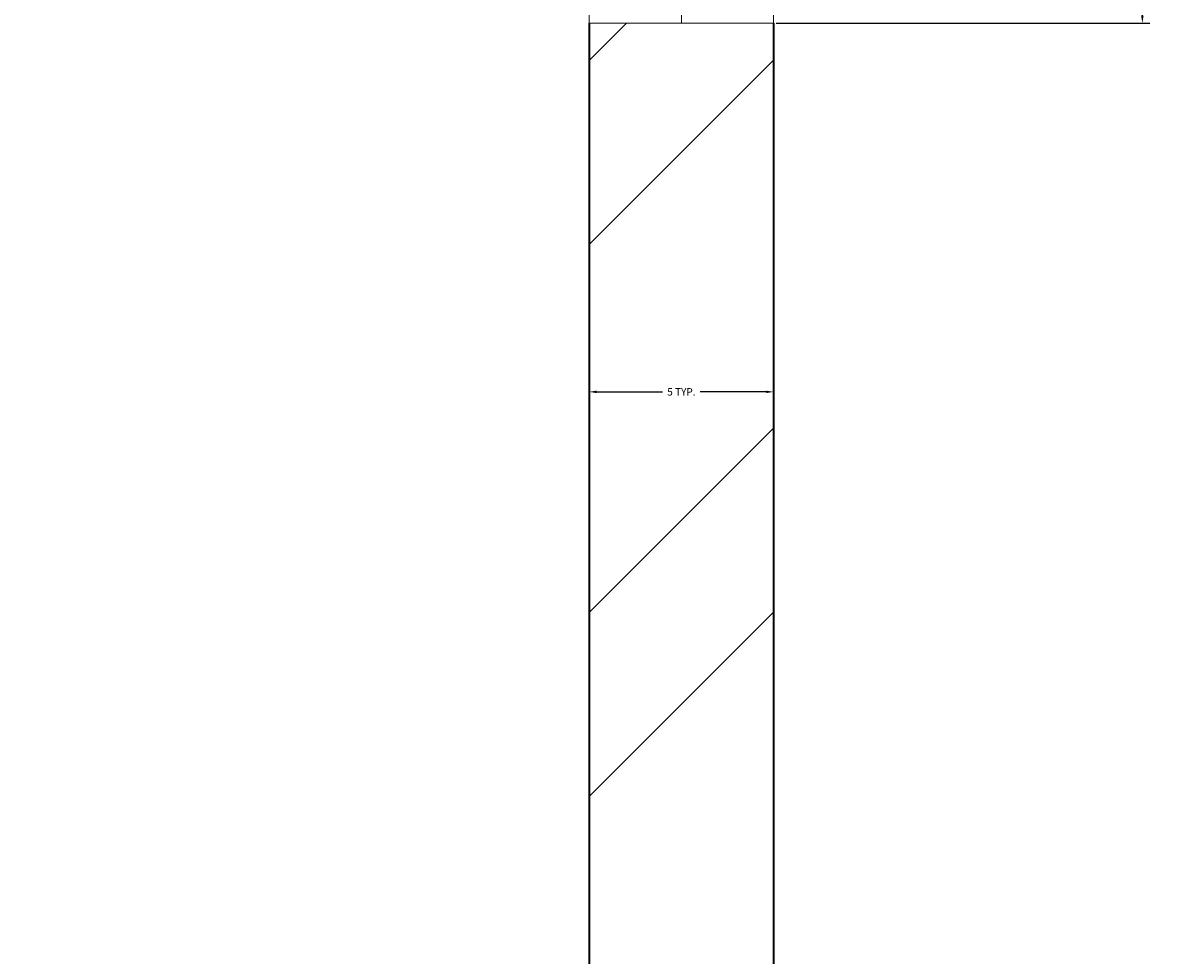
# Model space of a CAD drawing. Units: inches. Extents: x 2168 to 3056, y 1130 to 2629.
# Tile 41 of 42: x 2846 to 2874, y 2286 to 2308. Entities that reach past the tile are written whole.
import ezdxf

# ---------------------------------------------------------------- set-up
doc = ezdxf.new("R2010")
doc.units = ezdxf.units.IN
for name, color, linetype, lineweight in [('A-ANNO-DIMS', 2, 'Continuous', 18), ('A-GLAZ', 201, 'Continuous', 18), ('A-WALL', 7, 'Continuous', 35)]:
    doc.layers.add(name, color=color, linetype=linetype, lineweight=lineweight)
doc.layers.add('A-WALL-PATT', color=143, linetype='Continuous', lineweight=13, true_color=0x7aafdf)
doc.styles.get("Standard").update_dxf_attribs({"font": 'arial.ttf'})
doc.dimstyles.get("Standard").update_dxf_attribs({"dimtxt": 0.18, "dimasz": 0.18, "dimexe": 0.18, "dimexo": 0.0625, "dimgap": 0.09, "dimtad": 0, "dimtih": 1, "dimtoh": 1, "dimdec": 4, "dimzin": 0, "dimdsep": 46, "dimtxsty": 'Standard', "dimcen": 0.09, "dimadec": 0, "dimazin": 0, "dimtfac": 1, "dimtdec": 4, "dimtofl": 0, "dimtmove": 0, "dimatfit": 3, "dimfxl": 1, "dimtolj": 1, "dimtzin": 0, "dimarcsym": 0})

# ---------------------------------------------------------------- blocks, each defined once
blk = doc.blocks.new('WIN-60')
for p, q in [((0, 0), (0, 60)), ((2.25, 0), (2.25, 60)), ((4.5, 60), (4.5, 0)), ((0, 0), (4.5, 0)), ((4.5, 0), (2.25, 0))]:
    blk.add_line(p, q)
blk = doc.blocks.new('*D38')
at = {"layer": 'A-ANNO-DIMS', "color": 0, "lineweight": -2, "transparency": 16777216}
for p, q in [((2864.358, 2368.425), (2873.476, 2368.425)), ((2873.296, 2368.245), (2873.296, 2338.609)), ((2873.296, 2308.605), (2873.296, 2338.242)), ((2864.358, 2308.425), (2873.476, 2308.425))]:
    blk.add_line(p, q, dxfattribs=at)
at = {"layer": 'A-ANNO-DIMS', "color": 0, "transparency": 16777216}
for points in [[(2873.266, 2368.245), (2873.326, 2368.245), (2873.296, 2368.425)], [(2873.266, 2308.605), (2873.326, 2308.605), (2873.296, 2308.425)]]:
    blk.add_solid(points, dxfattribs=at)
at = {"layer": 'Defpoints', "color": 0, "transparency": 16777216}
for p in [(2864.296, 2368.425), (2873.296, 2368.425), (2864.296, 2308.425)]:
    blk.add_point(p, dxfattribs=at)
at = {"layer": 'A-ANNO-DIMS', "color": 0, "transparency": 16777216, "insert": (2873.296, 2338.425), "char_height": 0.18, "attachment_point": 5}
blk.add_mtext('\\A1;WINDOW 60 TYP.', dxfattribs=at)
blk = doc.blocks.new('*D39')
at = {"layer": 'A-ANNO-DIMS', "color": 0, "lineweight": -2, "transparency": 16777216}
for p, q in [((2859.796, 2308.363), (2859.796, 2299.245)), ((2864.296, 2308.363), (2864.296, 2299.245)), ((2859.976, 2299.425), (2861.588, 2299.425)), ((2864.116, 2299.425), (2862.504, 2299.425))]:
    blk.add_line(p, q, dxfattribs=at)
at = {"layer": 'A-ANNO-DIMS', "color": 0, "transparency": 16777216}
for points in [[(2859.976, 2299.455), (2859.976, 2299.395), (2859.796, 2299.425)], [(2864.116, 2299.455), (2864.116, 2299.395), (2864.296, 2299.425)]]:
    blk.add_solid(points, dxfattribs=at)
at = {"layer": 'Defpoints', "color": 0, "transparency": 16777216}
for p in [(2859.796, 2308.425), (2864.296, 2308.425), (2864.296, 2299.425)]:
    blk.add_point(p, dxfattribs=at)
at = {"layer": 'A-ANNO-DIMS', "color": 0, "transparency": 16777216, "insert": (2862.046, 2299.425), "char_height": 0.18, "attachment_point": 5}
blk.add_mtext('\\A1;5 TYP.', dxfattribs=at)

msp = doc.modelspace()

# ---------------------------------------------------------------- hatches: boundary and pattern name
at = {"layer": 'A-WALL-PATT'}
h = msp.add_hatch(dxfattribs=at)
h.set_pattern_fill('ANSI32', color=256)
h.paths.add_polyline_path([(2463.796, 2409.389), (2467.387, 2409.389), (2467.387, 2413.889), (2454.768, 2413.889), (2454.768, 2411.639), (2454.768, 2409.389), (2459.296, 2409.389), (2459.296, 2265.389), (2455.644, 2265.389), (2455.644, 2260.889), (2467.349, 2260.889), (2467.349, 2263.139), (2467.349, 2265.389), (2463.796, 2265.389)])
h.paths.add_polyline_path([(2431.596, 2413.889), (2409.647, 2413.889), (2409.647, 2409.389), (2431.596, 2409.389), (2431.596, 2411.639)])
h.paths.add_polyline_path([(2349.647, 2413.889), (2331.796, 2413.889), (2331.796, 2362.671), (2336.296, 2362.671), (2336.296, 2409.389), (2349.647, 2409.389), (2349.647, 2411.639)])
h.paths.add_polyline_path([(2634.149, 2411.639), (2634.149, 2413.889), (2562.293, 2413.889), (2562.293, 2409.389), (2595.796, 2409.389), (2595.796, 2280.309), (2595.826, 2280.309), (2595.826, 2265.389), (2499.91, 2265.389), (2499.91, 2260.889), (2550.796, 2260.889), (2550.796, 2117.308), (2555.296, 2117.308), (2555.296, 2168.08), (2571.93, 2168.08), (2571.93, 2176.889), (2559.796, 2176.889), (2559.796, 2256.389), (2640.796, 2256.389), (2640.796, 2176.889), (2626.428, 2176.889), (2626.428, 2168.08), (2645.296, 2168.08), (2645.296, 2116.637), (2649.796, 2116.637), (2649.796, 2260.889), (2691.251, 2260.889), (2691.251, 2263.139), (2691.251, 2265.389), (2670.655, 2265.389), (2670.655, 2265.365), (2600.296, 2265.365), (2600.296, 2280.258), (2600.296, 2409.389), (2634.149, 2409.389)])
h.paths.add_polyline_path([(2600.296, 2473.889), (2612.84, 2473.889), (2612.84, 2478.389), (2572.636, 2478.389), (2572.636, 2473.889), (2595.796, 2473.889), (2595.796, 2413.889), (2600.296, 2413.889)])
h.paths.add_polyline_path([(2535.796, 2473.889), (2548.636, 2473.889), (2548.636, 2478.389), (2531.396, 2478.389), (2531.396, 2413.889), (2521.6, 2413.889), (2521.6, 2409.389), (2539.239, 2409.389), (2539.239, 2411.639), (2539.239, 2413.889), (2535.796, 2413.889)])
h.paths.add_polyline_path([(2664.796, 2478.389), (2636.84, 2478.389), (2636.84, 2473.889), (2660.296, 2473.889), (2660.296, 2413.889), (2656.165, 2413.889), (2656.165, 2409.389), (2671.684, 2409.389), (2671.684, 2411.639), (2671.684, 2413.889), (2664.796, 2413.889)])
h.paths.add_polyline_path([(2705.942, 2413.889), (2695.684, 2413.889), (2695.684, 2409.389), (2705.942, 2409.389)])
h.paths.add_polyline_path([(2741.35, 2413.889), (2728.733, 2413.889), (2728.733, 2411.639), (2728.733, 2409.389), (2732.296, 2409.389), (2732.296, 2265.389), (2725.733, 2265.389), (2725.733, 2260.889), (2740.917, 2260.889), (2740.917, 2263.139), (2740.917, 2265.389), (2736.796, 2265.389), (2736.796, 2409.389), (2741.35, 2409.389)])
h.paths.add_polyline_path([(2785.655, 2413.889), (2764.546, 2413.889), (2764.486, 2409.389), (2785.655, 2409.389), (2785.655, 2411.639)])
h.paths.add_polyline_path([(2864.296, 2413.889), (2845.655, 2413.889), (2845.655, 2409.389), (2859.796, 2409.389), (2859.796, 2368.425), (2864.296, 2368.425)])
h.paths.add_polyline_path([(2864.296, 2308.425), (2862.046, 2308.425), (2859.796, 2308.425), (2859.796, 2265.389), (2774.483, 2265.389), (2774.483, 2263.139), (2774.483, 2260.889), (2781.796, 2260.889), (2781.796, 2226.654), (2786.296, 2226.654), (2786.296, 2260.889), (2859.796, 2260.889), (2859.796, 2241.352), (2864.296, 2241.352)])
h.paths.add_polyline_path([(2864.296, 2217.352), (2862.046, 2217.352), (2859.796, 2217.352), (2859.796, 2200.889), (2786.296, 2200.889), (2786.296, 2205.931), (2784.046, 2205.931), (2781.796, 2205.931), (2781.796, 2150.974), (2786.296, 2150.974), (2786.296, 2161.889), (2859.796, 2161.889), (2859.796, 2144.419), (2864.296, 2144.419)])
h.paths.add_polyline_path([(2859.796, 2196.389), (2859.796, 2166.389), (2786.296, 2166.389), (2786.296, 2196.389)], flags=16)
h.paths.add_polyline_path([(2864.296, 2108.419), (2862.046, 2108.419), (2859.796, 2108.419), (2859.796, 2080.889), (2786.296, 2080.889), (2786.296, 2111.993), (2781.796, 2111.993), (2781.796, 2080.889), (2649.796, 2080.889), (2649.796, 2086.036), (2647.546, 2086.036), (2645.296, 2086.036), (2645.296, 2071.739), (2649.796, 2071.739), (2649.796, 2076.389), (2781.796, 2076.389), (2781.796, 2041.792), (2786.296, 2041.792), (2786.296, 2076.389), (2859.796, 2076.389), (2859.796, 2058.577), (2864.296, 2058.577)])
h.paths.add_polyline_path([(2864.296, 2022.577), (2859.796, 2022.577), (2859.796, 1992.389), (2786.296, 1992.389), (2786.296, 1999.573), (2781.796, 1999.573), (2781.796, 1848.085), (2784.046, 1848.085), (2786.296, 1848.085), (2786.296, 1851.389), (2859.796, 1851.389), (2859.796, 1838.258), (2864.296, 1838.258)], flags=17)
h.paths.add_polyline_path([(2859.796, 1987.889), (2859.796, 1855.889), (2786.296, 1855.889), (2786.296, 1987.889)], flags=16)
h.paths.add_polyline_path([(2823.046, 1987.889), (2841.421, 1921.889), (2823.046, 1855.889)], flags=0)
h.paths.add_polyline_path([(2864.296, 1814.258), (2859.796, 1814.258), (2859.796, 1791.389), (2786.296, 1791.389), (2786.296, 1825.658), (2784.046, 1825.658), (2781.796, 1825.658), (2781.796, 1791.389), (2720.155, 1791.389), (2720.155, 1791.265), (2649.796, 1791.265), (2649.796, 1806.159), (2649.796, 2038.983), (2647.546, 2038.983), (2645.296, 2038.983), (2645.296, 1783.925), (2649.796, 1783.925), (2649.796, 1786.889), (2781.796, 1786.889), (2781.796, 1746.789), (2786.296, 1746.789), (2786.296, 1786.889), (2859.796, 1786.889), (2859.796, 1770.083), (2864.296, 1770.083)])
h.paths.add_polyline_path([(2864.296, 1734.083), (2862.046, 1734.083), (2859.796, 1734.083), (2859.796, 1705.889), (2786.296, 1705.889), (2786.296, 1714.166), (2781.796, 1714.166), (2781.796, 1660.527), (2786.296, 1660.527), (2786.296, 1666.889), (2859.796, 1666.889), (2859.796, 1648.342), (2864.296, 1648.342)])
h.paths.add_polyline_path([(2786.296, 1701.389), (2859.796, 1701.389), (2859.796, 1671.389), (2786.296, 1671.389)], flags=16)
h.paths.add_polyline_path([(2649.796, 1756.576), (2647.546, 1756.576), (2645.296, 1756.576), (2645.296, 1606.889), (2555.296, 1606.889), (2555.296, 1749.513), (2553.046, 1749.513), (2550.796, 1749.513), (2550.796, 1606.889), (2503.006, 1606.889), (2503.006, 1604.639), (2503.006, 1602.389), (2595.796, 1602.389), (2595.849, 1602.389), (2595.849, 1587.495), (2595.796, 1458.389), (2561.502, 1458.389), (2561.502, 1456.139), (2561.502, 1453.889), (2595.796, 1453.889), (2595.796, 1381.889), (2573.438, 1381.889), (2573.438, 1377.389), (2613.01, 1377.389), (2613.01, 1379.639), (2613.01, 1381.889), (2600.296, 1381.889), (2600.296, 1453.889), (2634.327, 1453.889), (2634.327, 1458.389), (2600.296, 1458.389), (2600.296, 1602.389), (2670.655, 1602.389), (2694.095, 1602.389), (2694.095, 1606.889), (2649.796, 1606.889)])
h.paths.add_polyline_path([(2736.796, 1602.389), (2741.562, 1602.389), (2741.562, 1606.889), (2726.203, 1606.889), (2726.203, 1604.639), (2726.203, 1602.389), (2732.296, 1602.389), (2732.296, 1458.389), (2727.899, 1458.389), (2727.899, 1453.889), (2740.821, 1453.889), (2740.821, 1456.139), (2740.821, 1458.389), (2736.796, 1458.389)])
h.paths.add_polyline_path([(2859.796, 1606.889), (2786.296, 1606.889), (2786.296, 1637.334), (2784.046, 1637.334), (2781.796, 1637.334), (2781.796, 1606.889), (2775.612, 1606.889), (2775.612, 1602.389), (2859.796, 1602.389)])
h.paths.add_polyline_path([(2864.296, 1624.342), (2862.046, 1624.342), (2859.796, 1624.342), (2859.796, 1570.39), (2864.296, 1570.39)])
h.paths.add_polyline_path([(2864.296, 1510.39), (2862.046, 1510.39), (2859.796, 1510.39), (2859.796, 1458.389), (2846.735, 1458.389), (2846.735, 1456.139), (2846.735, 1453.889), (2864.296, 1453.889)])
h.paths.add_polyline_path([(2786.735, 1458.389), (2765.444, 1458.389), (2765.444, 1453.889), (2786.735, 1453.889)])
h.paths.add_polyline_path([(2706.004, 1458.389), (2695.36, 1458.389), (2695.36, 1453.889), (2706.004, 1453.889), (2706.004, 1456.139)])
h.paths.add_polyline_path([(2671.36, 1456.139), (2671.36, 1458.389), (2655.986, 1458.389), (2655.986, 1456.139), (2655.986, 1453.889), (2660.296, 1453.889), (2660.296, 1381.889), (2637.01, 1381.889), (2637.01, 1377.389), (2664.796, 1377.389), (2664.796, 1453.889), (2671.36, 1453.889)], flags=17)
h.paths.add_polyline_path([(2539.829, 1458.389), (2520.237, 1458.389), (2520.237, 1453.889), (2531.296, 1453.889), (2531.296, 1377.389), (2546.449, 1377.389), (2546.449, 1379.639), (2546.449, 1381.889), (2535.796, 1381.889), (2535.796, 1453.889), (2539.829, 1453.889)], flags=17)
h.paths.add_polyline_path([(2496.237, 1458.389), (2489.13, 1458.389), (2489.13, 1453.889), (2496.237, 1453.889), (2496.237, 1456.139)])
h.paths.add_polyline_path([(2467.433, 1456.139), (2467.433, 1458.389), (2463.796, 1458.389), (2463.796, 1602.389), (2468.242, 1602.389), (2468.242, 1605.7), (2468.242, 1606.889), (2454.602, 1606.889), (2454.602, 1602.389), (2459.296, 1602.389), (2459.296, 1458.389), (2454.24, 1458.389), (2454.24, 1453.889), (2467.433, 1453.889)])
h.paths.add_polyline_path([(2431.601, 1456.139), (2431.601, 1458.389), (2411.386, 1458.389), (2411.386, 1453.889), (2431.601, 1453.889)])
h.paths.add_polyline_path([(2351.386, 1458.389), (2336.296, 1458.389), (2336.296, 1490.693), (2334.046, 1490.693), (2331.796, 1490.693), (2331.796, 1453.889), (2351.386, 1453.889), (2351.386, 1456.139)])
h.paths.add_polyline_path([(2336.296, 1629.705), (2331.796, 1629.705), (2331.796, 1552.317), (2336.296, 1552.317), (2336.296, 1602.389), (2406.655, 1602.389), (2423.472, 1602.389), (2423.472, 1606.889), (2418.796, 1606.889), (2418.796, 1643.678), (2416.546, 1643.678), (2414.296, 1643.678), (2414.296, 1606.889), (2336.296, 1606.889)])
h.paths.add_polyline_path([(2418.796, 1714.384), (2414.296, 1714.384), (2414.296, 1705.889), (2336.296, 1705.889), (2336.296, 1731.324), (2334.046, 1731.324), (2331.796, 1731.324), (2331.796, 1653.705), (2334.046, 1653.705), (2336.296, 1653.705), (2336.296, 1666.889), (2414.296, 1666.889), (2414.296, 1663.589), (2418.796, 1663.589)])
h.paths.add_polyline_path([(2336.296, 1701.389), (2414.296, 1701.389), (2414.296, 1671.389), (2336.296, 1671.389)], flags=16)
h.paths.add_polyline_path([(2555.296, 2040.059), (2550.796, 2040.059), (2550.796, 1791.389), (2550.561, 1791.205), (2480.202, 1791.205), (2418.796, 1791.389), (2418.796, 1825.448), (2416.546, 1825.448), (2414.296, 1825.448), (2414.296, 1791.389), (2336.296, 1791.389), (2336.296, 1806.409), (2331.796, 1806.409), (2331.796, 1767.324), (2336.296, 1767.324), (2336.296, 1786.889), (2414.296, 1786.889), (2414.296, 1745.457), (2418.796, 1745.457), (2418.796, 1786.889), (2550.796, 1786.889), (2550.796, 1783.011), (2555.296, 1783.011)])
h.paths.add_polyline_path([(2418.796, 1923.389), (2423.207, 1923.389), (2423.207, 1925.639), (2423.207, 1927.889), (2418.796, 1927.889), (2418.796, 2000.048), (2414.296, 2000.048), (2414.296, 1992.389), (2336.296, 1992.389), (2336.296, 1987.889), (2414.296, 1987.889), (2414.296, 1855.889), (2336.296, 1855.889), (2336.296, 1851.389), (2414.296, 1851.389), (2414.296, 1846.759), (2418.796, 1846.759)], flags=17)
h.paths.add_polyline_path([(2336.296, 2019.294), (2334.046, 2019.294), (2331.796, 2019.294), (2331.796, 1830.409), (2336.296, 1830.409)], flags=17)
h.paths.add_polyline_path([(2550.796, 1927.889), (2453.541, 1927.889), (2453.541, 1925.639), (2453.541, 1923.389), (2550.796, 1923.389)], flags=17)
h.paths.add_polyline_path([(2744.987, 1927.889), (2649.796, 1927.889), (2649.796, 1923.389), (2744.987, 1923.389), (2744.987, 1925.639)], flags=17)
h.paths.add_polyline_path([(2555.296, 2086.458), (2553.046, 2086.458), (2550.796, 2086.458), (2550.796, 2080.889), (2418.796, 2080.889), (2336.296, 2080.889), (2336.296, 2115.399), (2334.046, 2115.399), (2331.796, 2115.399), (2331.796, 2055.294), (2336.296, 2055.294), (2336.296, 2076.389), (2550.796, 2076.389), (2550.796, 2071.538), (2555.296, 2071.538)])
h.paths.add_polyline_path([(2418.796, 2121.389), (2414.296, 2121.389), (2414.296, 2080.889), (2418.796, 2080.889)])
h.paths.add_polyline_path([(2418.796, 2076.389), (2414.296, 2076.389), (2414.296, 2035.123), (2418.796, 2035.123)])
h.paths.add_polyline_path([(2422.868, 2263.139), (2422.868, 2265.389), (2406.655, 2265.389), (2406.655, 2265.359), (2336.296, 2265.359), (2336.296, 2280.252), (2336.296, 2302.671), (2334.046, 2302.671), (2331.796, 2302.671), (2331.796, 2246.853), (2336.296, 2246.853), (2336.296, 2260.889), (2414.296, 2260.889), (2414.296, 2223.996), (2418.796, 2223.996), (2418.796, 2260.889), (2422.868, 2260.889)])
h.paths.add_polyline_path([(2418.796, 2204.783), (2416.546, 2204.783), (2414.296, 2204.783), (2414.296, 2200.889), (2336.296, 2200.889), (2336.296, 2220.853), (2331.796, 2220.853), (2331.796, 2151.399), (2336.296, 2151.399), (2336.296, 2161.889), (2414.296, 2161.889), (2414.296, 2153.726), (2418.796, 2153.726)])
h.paths.add_polyline_path([(2414.296, 2196.389), (2414.296, 2166.389), (2336.296, 2166.389), (2336.296, 2196.389)], flags=16)
h.paths.add_polyline_path([(2375.296, 2181.389), (2336.296, 2166.389), (2336.296, 2196.389)], flags=0)
h.paths.add_polyline_path([(2809.595, 2172.34), (2838.804, 2172.34), (2838.804, 2190.997), (2809.595, 2190.997)], flags=8)
h.paths.add_polyline_path([(2849.75, 1919.585), (2849.75, 1952.672), (2831.093, 1952.672), (2831.093, 1919.585)], flags=8)
h.paths.add_polyline_path([(2808.875, 1901.967), (2808.875, 1937.85), (2790.149, 1937.85), (2790.149, 1901.967)], flags=8)
h.paths.add_polyline_path([(2806.285, 1671.896), (2835.493, 1671.896), (2835.493, 1690.553), (2806.285, 1690.553)], flags=8)
h.paths.add_polyline_path([(2353.186, 1676.549), (2382.395, 1676.549), (2382.395, 1695.207), (2353.186, 1695.207)], flags=8)
h.paths.add_polyline_path([(2360.083, 1832.308), (2389.241, 1832.308), (2389.241, 1850.966), (2360.083, 1850.966)], flags=25)
h.paths.add_polyline_path([(2354.822, 2167.823), (2384.031, 2167.823), (2384.031, 2186.481), (2354.822, 2186.481)], flags=8)

# ---------------------------------------------------------------- linework, layer by layer
at = {"layer": 'A-WALL'}
for p, q in [((2859.796, 2308.425), (2859.796, 2265.389)), ((2864.296, 2308.425), (2864.296, 2241.352))]:
    msp.add_line(p, q, dxfattribs=at)

# ---------------------------------------------------------------- block references
at = {"layer": 'A-GLAZ'}
msp.add_blockref('WIN-60', (2859.796, 2308.425), dxfattribs=at)

# ---------------------------------------------------------------- dimensions: what is measured, and where the dimension line sits
at = {"layer": 'A-ANNO-DIMS'}
dim = msp.add_linear_dim(base=(2873.296, 2368.425), p1=(2864.296, 2308.425), p2=(2864.296, 2368.425), angle=90, text='WINDOW <> TYP.', dimstyle='Standard', override={"dimdec": 0, "dimlfac": 1, "dimrnd": 0, "dimzin": 0, "dimdsep": 46, "dimlunit": 2}, dxfattribs=at)
dim.commit()
dim.dimension.update_dxf_attribs({"geometry": '*D38', "text_midpoint": (2873.296, 2338.425)})
dim = msp.add_linear_dim(base=(2864.29575579, 2299.425486635), p1=(2859.79575579, 2308.425486635), p2=(2864.29575579, 2308.425486635), text='<> TYP.', dimstyle='Standard', override={"dimdec": 0, "dimlfac": 1, "dimrnd": 0, "dimzin": 0, "dimdsep": 46, "dimlunit": 2}, dxfattribs=at)
dim.commit()
dim.dimension.update_dxf_attribs({"geometry": '*D39', "text_midpoint": (2862.04575579, 2299.425486635)})

doc.saveas('drawing.dxf')
